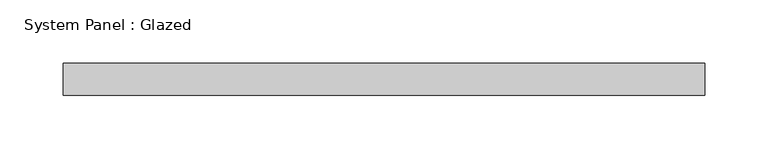
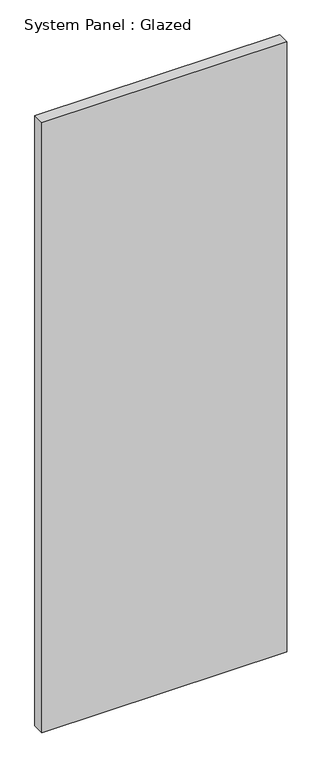
"""IFC4 building model written with IfcOpenShell, lengths in millimetres: plate geometry, System Panel : Glazed."""

from ifc_helpers import new_model, si_unit, origin, origin_with_axes, place, context, project, spatial, polyline, outline, extrude, source, transform, mapped, element, save


def system_panel_glazed_14783ebf(model_context):
    return source(origin(), model_context, "Body", "SweptSolid", [
        extrude(outline(polyline([(253.4574609, 19.05), (-253.4574609, 19.05), (-253.4574609, 44.45), (253.4574609, 44.45), (253.4574609, 19.05)])), origin_with_axes(), (0.0, 0.0, 1.0), 1336.1285226),
    ])


if __name__ == "__main__":
    model = new_model("IFC4")
    model_context = context("Model", 3, world=origin())
    ifc_project = project(units=[si_unit("LENGTHUNIT", "METRE", prefix="MILLI")], contexts=[model_context])
    site = spatial("IfcSite", under=ifc_project)
    building = spatial("IfcBuilding", under=site)
    placement = place(None, origin())
    system_panel_glazed_shape = system_panel_glazed_14783ebf(model_context)
    element("IfcPlate", 1, ObjectType="System Panel : Glazed", at=placement, inside=building, context=model_context, shape_type="MappedRepresentation", body=[
        mapped(system_panel_glazed_shape, transform((0.0, 0.0, 0.0), x_axis=(1.0, 0.0, 0.0), y_axis=(0.0, 1.0, 0.0), z_axis=(0.0, 0.0, 1.0))),
    ])
    save(model, "model.ifc")

# Revit data of these elements
# Type "System Panel : Glazed"
#   Construction Type Id = "GSP4R"
#   Analytic Construction = "1/8 in Pilkington single glazing"
#   Visual Light Transmittance = 0.9
#   Solar Heat Gain Coefficient = 0.86
#   Heat Transfer Coefficient (U) = 1.18115 BTU/(h·ft²·°F)
#   Define Thermal Properties by = 1
# Element 1 (IfcPlate, "System Panel : Glazed")
#   Materials on its faces: "Glass"
# Materials
#   "Glass": class "Glass", colour RGB 0 128 192, transparency 0.75, Description = "Soda Lime Glass", Cost = 0
